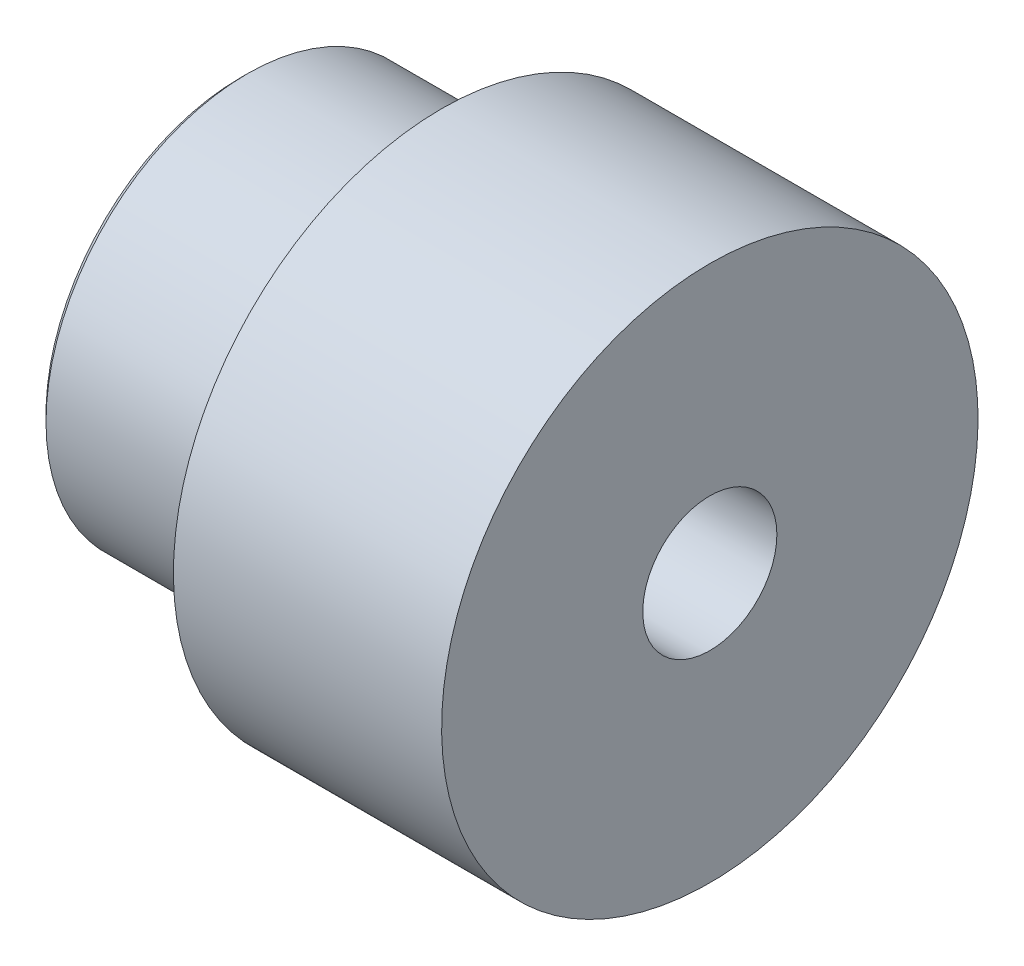
from build123d import *

# Parameters (mm, degrees)
EDGE_CHAMFER_0_025IN_X_45DEG_SIZE  = 0.635
DRILLED_HOLE_0_5_X_0_75_DEEP_D     = 12.7
DRILLED_HOLE_0_5_X_0_75_DEEP_DEPTH = 19.05
DRILLED_HOLE_0_5_X_0_75_DEEP_TIP   = 3.815464931


with BuildPart() as part:
    # Turned Profile Sketch → Turned Body (revolve)
    with BuildSketch(Plane.XY):
        Polygon((0, 0), (0, 25.4), (-25.4, 25.4), (-25.4, 19.05), (-44.45, 19.05), (-44.45, 0), (-0.941021968, 0), align=None)
    revolve(axis=Axis((-0.941021968, 0, 0), (-1, 0, 0)))

    # Sketch4 → Tapped Hole 1-4-20 x 0.5 Deep (revolve, cut)
    with BuildSketch(Plane(origin=(-44.45, 0, 0), x_dir=(0, 0, 1), z_dir=(0, 1, 0))):
        Polygon((0, 0), (0, 20.583816902), (2.5527, 19.05), (2.5527, 12.7), (3.175, 12.7), (3.175, 0.730483939), (3.81, 0), align=None)
    revolve(axis=Axis((-50.8, 0, 0), (1, 0, 0)), mode=Mode.SUBTRACT)

    # Edge Chamfer 0.025in x 45deg
    edge_chamfer_0_025in_x_45deg_edges = [part.edges().sort_by_distance(p)[0] for p in [
        (-44.45, -19.05, 0),
    ]]
    chamfer(edge_chamfer_0_025in_x_45deg_edges, length=EDGE_CHAMFER_0_025IN_X_45DEG_SIZE)

    # Drilled Hole Ø0.5 x 0.75 Deep
    with Locations(Plane.YZ):
        with Locations((0, 0)):
            Hole(DRILLED_HOLE_0_5_X_0_75_DEEP_D / 2, depth=DRILLED_HOLE_0_5_X_0_75_DEEP_DEPTH)
            with Locations((0, 0, -(DRILLED_HOLE_0_5_X_0_75_DEEP_DEPTH + DRILLED_HOLE_0_5_X_0_75_DEEP_TIP / 2))):  # 118° drill point
                Cone(0, DRILLED_HOLE_0_5_X_0_75_DEEP_D / 2, DRILLED_HOLE_0_5_X_0_75_DEEP_TIP, mode=Mode.SUBTRACT)


solid = part.part
